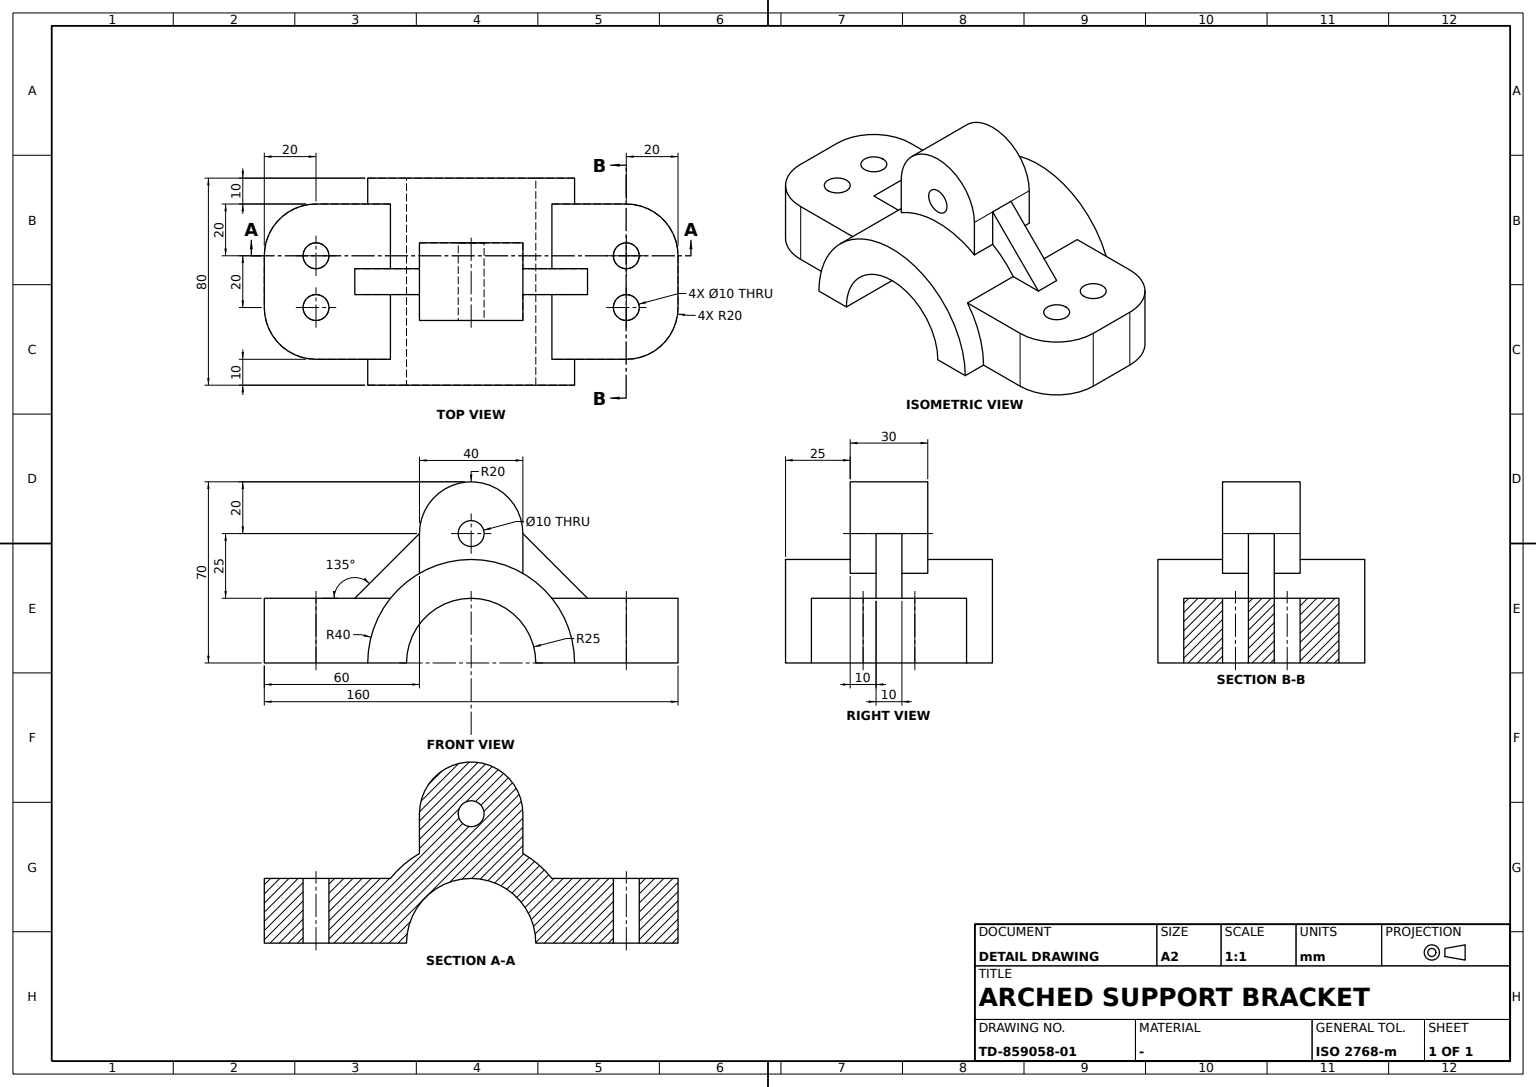
CATIA V5 part; units mm, degrees
sketch "Sketch1" plane through (0, 0, 0) normal (1, 0, 0) x (0, 1, 0)
  line L0 (-80, 0) -> (80, 0)
  line L1 (80, 0) -> (80, 25)
  line L2 (-80, 0) -> (-80, 25)
  line L3 (-80, 25) -> (-31.225, 25)
  line L4 (80, 25) -> (31.225, 25)
  line L5 (-31.225, 25) -> (31.225, 25)
  dimension "length L0" = 160
  dimension "length L1" = 25
  dimension "length L2" = 25
  dimension "length L4" = 48.775
  dimension "length L3" = 48.775
  dimension "length L5" = 62.45
  constraint midpoint L0 origin
  constraint horizontal L0 x-axis
  constraint horizontal L5 x-axis
  constraint vertical L1 y-axis
  constraint vertical L2 y-axis
extrude "Pad1" add sketch "Sketch1" along normal mid plane 60
sketch "Sketch2" plane through (0, 0, 0) normal (1, 0, 0) x (0, 1, 0)
  arc A0 (40, 0) -> (-40, 0) centre (0, 0) ccw
  point P0 (40, 0)
  line L0 (-40, 0) -> (40, 0)
  dimension "radius A0" = 40
  constraint coincidence P0 x-axis
  constraint horizontal L0 x-axis
extrude "Pad2" add sketch "Sketch2" along normal mid plane 80
sketch "Sketch3" plane through (40, 0, 0) normal (1, 0, 0) x (0, 1, 0)
  circle A0 centre (0, 0) radius 25
  dimension "radius A0" = 25
extrude "Pocket1" cut sketch "Sketch3" against normal through all
sketch "Sketch4" plane through (0, 0, 0) normal (1, 0, 0) x (0, 1, 0)
  line L0 (-20, 50) -> (-20, 34.641)
  point P0 (-20, 50)
  point P1 (-20, 34.641)
  arc A0 (40, 0) -> (-40, 0) centre (0, 0) ccw construction
  line L1 (20, 50) -> (20, 34.641)
  point P2 (20, 50)
  point P3 (20, 34.641)
  arc A1 (-20, 50) -> (20, 50) centre (0, 50) cw
  arc A2 (20, 34.641) -> (-20, 34.641) centre (0, 0) ccw
  dimension "distance L0 y axis" = 20
  dimension "distance P0 x axis" = 50
  dimension "distance L1 y axis" = 20
  dimension "distance P2 x axis" = 50
  constraint vertical L0 y-axis
  constraint vertical L1 y-axis
  constraint coincidence P1 A0
  constraint coincidence P3 A0
  constraint tangency A1 L1
extrude "Pad3" add sketch "Sketch4" along normal mid plane 30
sketch "Sketch5" plane through (15, 0, 0) normal (1, 0, 0) x (0, 1, 0)
  circle A0 centre (0, 50) radius 5
  arc A1 (20, 50) -> (-20, 50) centre (0, 50) ccw construction
  dimension "radius A0" = 5
  constraint concentricity A0 A1
extrude "Pocket2" cut sketch "Sketch5" against normal through all
fillet "Fillet1" radius 20 2 edges at (30, 80, 12.5) (-30, 80, 12.5)
fillet "Fillet2" radius 20 1 edges at (30, -80, 12.5)
fillet "Fillet3" radius 20 1 edges at (-30, -80, 12.5)
sketch "Sketch6" plane through (0, 0, 25) normal (0, 0, 1) x (1, 0, 0)
  circle A0 centre (-10, 60) radius 5
  point P0 (-10, 60)
  circle A1 centre (10, 60) radius 5
  point P1 (10, 60)
  dimension "radius A0" = 5
  dimension "distance P0 x axis" = 60
  dimension "distance P0 y axis" = 10
  dimension "radius A1" = 5
  dimension "distance P1 y axis" = 10
  dimension "D6" = 60
extrude "Pocket3" cut sketch "Sketch6" against normal through all
sketch "Sketch7" plane through (0, 0, 25) normal (0, 0, 1) x (1, 0, 0)
  circle A0 centre (-10, -60) radius 5
  point P0 (-10, -60)
  circle A1 centre (10, -60) radius 5
  point P1 (10, -60)
  dimension "radius A0" = 5
  dimension "distance P0 x axis" = 60
  dimension "distance P0 y axis" = 10
  dimension "radius A1" = 5
  dimension "distance P1 x axis" = 60
  dimension "distance P1 y axis" = 10
extrude "Pocket4" cut sketch "Sketch7" against normal through all
sketch "Sketch8" plane through (0, 0, 0) normal (1, 0, 0) x (0, 1, 0)
  line L0 (20, 50) -> (45, 25)
  point P0 (20, 50)
  point P1 (45, 25)
  point P2 (20, 50)
  line L1 (80, 25) -> (31.225, 25) construction
  dimension "distance P1 y axis" = 45
  constraint coincidence P0 P2
  constraint coincidence P1 L1
rib "Stiffener1" sketch "Sketch8" thickness 10 sides both
sketch "Sketch9" plane through (0, 0, 0) normal (1, 0, 0) x (0, 1, 0)
  line L0 (-20, 50) -> (-45, 25)
  point P0 (-20, 50)
  point P1 (-45, 25)
  point P2 (-20, 50)
  line L1 (-31.225, 25) -> (-80, 25) construction
  dimension "distance P1 y axis" = 45
  constraint coincidence P0 P2
  constraint coincidence P1 L1
rib "Stiffener2" sketch "Sketch9" thickness 10 sides both
